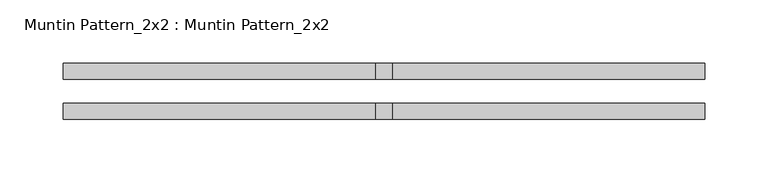
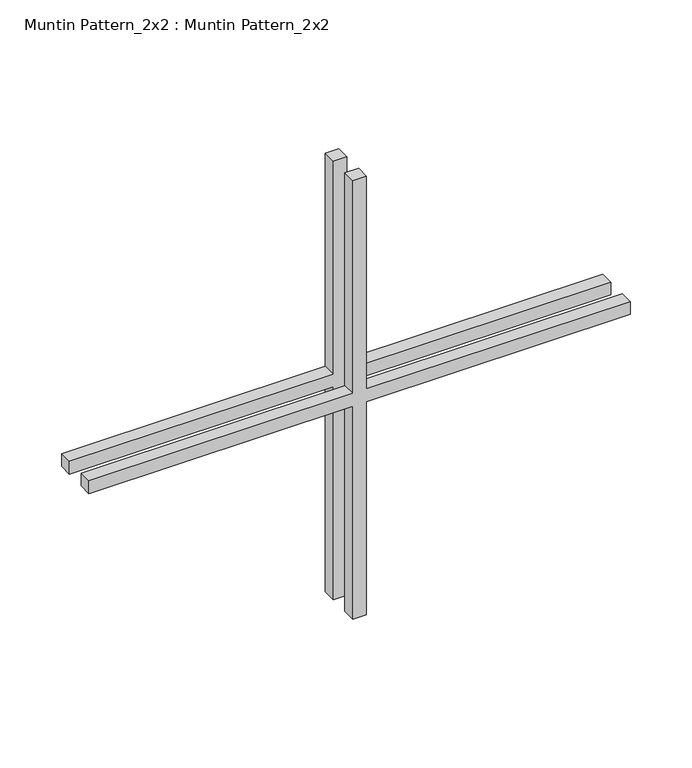
"""IFC4 building model written with IfcOpenShell, lengths in millimetres: proxy geometry, Muntin Pattern_2x2 : Muntin Pattern_2x2."""

from ifc_helpers import new_model, si_unit, frame, origin, place, context, project, spatial, polyline, outline, extrude, source, transform, mapped, element, save


def muntin_pattern_2x2_muntin_pattern_2x2_183aef24(model_context):
    return source(origin(), model_context, "Body", "SweptSolid", [
        extrude(outline(polyline([(223.8375, -6.35), (223.8375, -254.0), (211.1375, -254.0), (211.1375, -6.35), (0.0, -6.35), (0.0, 6.35), (211.1375, 6.35), (211.1375, 254.0), (223.8375, 254.0), (223.8375, 6.35), (434.975, 6.35), (434.975, -6.35), (223.8375, -6.35)])), frame((0.0, -22.225, 0.0), z_axis=(0.0, 1.0, 0.0), x_axis=(0.0, 0.0, 1.0)), (0.0, 0.0, 1.0), 12.7),
        extrude(outline(polyline([(223.8375, -6.35), (223.8375, -254.0), (211.1375, -254.0), (211.1375, -6.35), (0.0, -6.35), (0.0, 6.35), (211.1375, 6.35), (211.1375, 254.0), (223.8375, 254.0), (223.8375, 6.35), (434.975, 6.35), (434.975, -6.35), (223.8375, -6.35)])), frame((0.0, 9.525, 0.0), z_axis=(0.0, 1.0, 0.0), x_axis=(0.0, 0.0, 1.0)), (0.0, 0.0, 1.0), 12.7),
    ])


if __name__ == "__main__":
    model = new_model("IFC4")
    model_context = context("Model", 3, world=origin())
    ifc_project = project(units=[si_unit("LENGTHUNIT", "METRE", prefix="MILLI")], contexts=[model_context])
    site = spatial("IfcSite", under=ifc_project)
    building = spatial("IfcBuilding", under=site)
    placement = place(None, origin())
    muntin_pattern_2x2_muntin_pattern_2x2_shape = muntin_pattern_2x2_muntin_pattern_2x2_183aef24(model_context)
    element("IfcBuildingElementProxy", 1, Name="Muntin Pattern_2x2 : Muntin Pattern_2x2", ObjectType="Muntin Pattern_2x2 : Muntin Pattern_2x2", at=placement, inside=building, context=model_context, shape_type="MappedRepresentation", body=[
        mapped(muntin_pattern_2x2_muntin_pattern_2x2_shape, transform((0.0, 0.0, 0.0), x_axis=(1.0, 0.0, 0.0), y_axis=(0.0, 1.0, 0.0), z_axis=(0.0, 0.0, 1.0))),
    ])
    save(model, "model.ifc")

# Revit data of these elements
# Type "Muntin Pattern_2x2 : Muntin Pattern_2x2"
#   Width [instance default] = 4' - 0"
#   Thickness = 0' - 0 1/2"
#   Height [instance default] = 4' - 0"
#   Distance = 0' - 0 3/4"
#   Interior Material [instance default] = none
#   Exterior Material [instance default] = none
#   Default Elevation = 0
# Element 1 (IfcBuildingElementProxy, "Muntin Pattern_2x2 : Muntin Pattern_2x2")
#   Width = 1' - 8"
#   Height = 1' - 5 1/8"
#   Interior Material = Wood - Stained
#   Exterior Material = Clad - White
#   Materials on its faces: "Clad - White", "Wood - Stained"
# Materials
#   "Clad - White": class "Wood", colour RGB 242 242 238, transparency 0, Cost = 0
#   "Wood - Stained": class "Wood", colour RGB 224 178 126, transparency 0, Cost = 0
